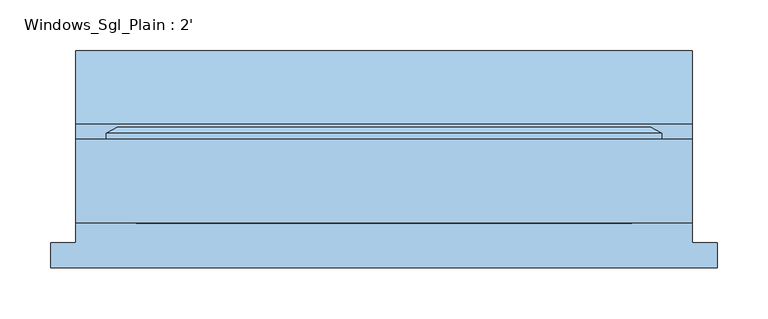
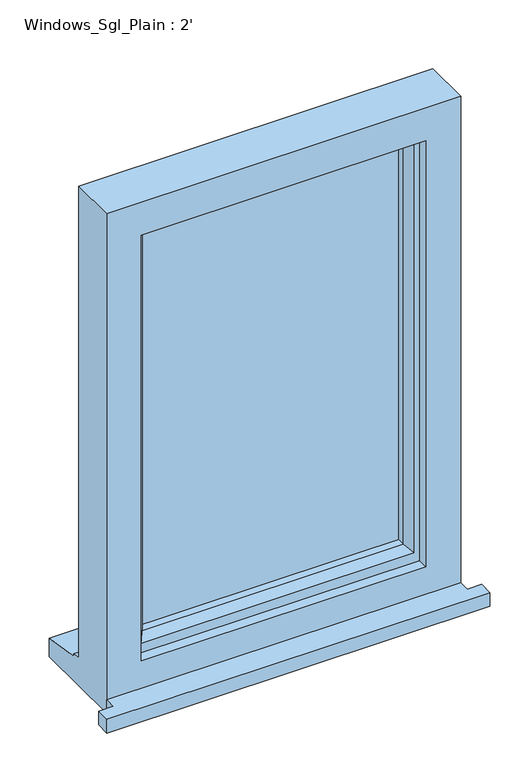
"""IFC4 building model written with IfcOpenShell, lengths in millimetres: window geometry, Windows_Sgl_Plain : 2'."""

from ifc_helpers import new_model, si_unit, frame, origin, place, context, project, spatial, polyline, outline, extrude, faceted_brep, source, transform, mapped, element, save


def windows_sgl_plain_2_be143095(model_context):
    return source(origin(), model_context, "Body", "SolidModel", [
        extrude(outline(polyline([(-329.8, -92.7434322), (-329.8, -67.7434322), (-304.8, -67.7434322), (-304.8, -48.3434322), (304.8, -48.3434322), (304.8, -67.7434322), (329.8, -67.7434322), (329.8, -92.7434322), (-329.8, -92.7434322)])), frame((0.0, 0.0, 1200.0), z_axis=(0.0, 0.0, 1.0), x_axis=(1.0, 0.0, 0.0)), (0.0, 0.0, 1.0), 25.0),
        faceted_brep([(-304.8, -48.3434322, 1200.0), (304.8, -48.3434322, 1200.0), (304.8, -48.3434322, 2110.0), (-304.8, -48.3434322, 2110.0), (-244.8, -48.3434322, 2050.0), (244.8, -48.3434322, 2050.0), (244.8, -48.3434322, 1275.0), (-244.8, -48.3434322, 1275.0), (-304.8, 34.6565678, 2110.0), (-304.8, 34.6565678, 1251.0), (-304.8, 49.6565678, 1249.68767), (-304.8, 49.6565678, 1244.7449676), (-304.8, 122.1565678, 1233.8088847), (-304.8, 122.1565678, 1200.0), (304.8, 34.6565678, 2110.0), (304.8, 34.6565678, 1251.0), (-264.8, 34.6565678, 2070.0), (-264.8, 34.6565678, 1263.0), (264.8, 34.6565678, 1263.0), (264.8, 34.6565678, 2070.0), (-264.8, -30.3434322, 2070.0), (-264.8, -30.3434322, 1263.0), (264.8, -30.3434322, 2070.0), (264.8, -30.3434322, 1263.0), (-244.8, -30.3434322, 2050.0), (-244.8, -30.3434322, 1275.0), (244.8, -30.3434322, 1275.0), (244.8, -30.3434322, 2050.0), (304.8, 122.1565678, 1200.0), (304.8, 122.1565678, 1233.8088847), (304.8, 49.6565678, 1244.7449676), (304.8, 49.6565678, 1249.68767)], [[[0, 1, 2, 3], [4, 5, 6, 7]], [[0, 3, 8, 9, 10, 11, 12, 13]], [[9, 8, 14, 15], [16, 17, 18, 19]], [[17, 16, 20, 21]], [[20, 22, 23, 21], [24, 25, 26, 27]], [[24, 4, 7, 25]], [[3, 2, 14, 8]], [[16, 19, 22, 20]], [[5, 4, 24, 27]], [[15, 14, 2, 1, 28, 29, 30, 31]], [[19, 18, 23, 22]], [[5, 27, 26, 6]], [[28, 1, 0, 13]], [[29, 28, 13, 12]], [[30, 29, 12, 11]], [[31, 30, 11, 10]], [[15, 31, 10, 9]], [[21, 23, 18, 17]], [[7, 6, 26, 25]]]),
        extrude(outline(polyline([(234.8, -1.3434322), (-234.8, -1.3434322), (-234.8, 22.6565678), (234.8, 22.6565678), (234.8, -1.3434322)])), frame((0.0, 0.0, 1293.0), z_axis=(0.0, 0.0, 1.0), x_axis=(1.0, 0.0, 0.0)), (0.0, 0.0, 1.0), 747.0),
        faceted_brep([(-274.8, 34.6565678, 2080.0), (-274.8, 40.4300705, 2080.0), (-274.8, 40.4300705, 1253.0), (-274.8, 34.6565678, 1253.0), (-264.8, -30.3434322, 2070.0), (-264.8, 34.6565678, 2070.0), (-264.8, 34.6565678, 1263.0), (-264.8, -30.3434322, 1263.0), (-224.8, -15.8505323, 2030.0), (-234.9480377, -30.3434322, 2040.1480377), (-234.9480377, -30.3434322, 1292.8519623), (-224.8, -15.8505323, 1303.0), (-224.8, -1.3434322, 2030.0), (-224.8, -1.3434322, 1303.0), (-234.8, 22.6565678, 2040.0), (-234.8, -1.3434322, 2040.0), (-234.8, -1.3434322, 1293.0), (-234.8, 22.6565678, 1293.0), (-224.8, 40.4300705, 2030.0), (-224.8, 22.6565678, 2030.0), (-224.8, 22.6565678, 1303.0), (-224.8, 40.4300705, 1303.0), (-242.2457548, 46.2035732, 2047.4457548), (-242.2457548, 46.2035732, 1285.5542452), (-264.0153903, 46.2035732, 2069.2153903), (-264.0153903, 46.2035732, 1263.7846097), (274.8, 40.4300705, 1253.0), (274.8, 34.6565678, 1253.0), (264.8, 34.6565678, 1263.0), (264.8, -30.3434322, 1263.0), (234.9480377, -30.3434322, 1292.8519623), (224.8, -15.8505323, 1303.0), (224.8, -1.3434322, 1303.0), (234.8, -1.3434322, 1293.0), (234.8, 22.6565678, 1293.0), (224.8, 22.6565678, 1303.0), (224.8, 40.4300705, 1303.0), (242.2457548, 46.2035732, 1285.5542452), (264.0153903, 46.2035732, 1263.7846097), (274.8, 40.4300705, 2080.0), (274.8, 34.6565678, 2080.0), (264.8, 34.6565678, 2070.0), (264.8, -30.3434322, 2070.0), (234.9480377, -30.3434322, 2040.1480377), (224.8, -15.8505323, 2030.0), (224.8, -1.3434322, 2030.0), (234.8, -1.3434322, 2040.0), (234.8, 22.6565678, 2040.0), (224.8, 22.6565678, 2030.0), (224.8, 40.4300705, 2030.0), (242.2457548, 46.2035732, 2047.4457548), (264.0153903, 46.2035732, 2069.2153903)], [[[0, 1, 2, 3]], [[4, 5, 6, 7]], [[8, 9, 10, 11]], [[12, 8, 11, 13]], [[14, 15, 16, 17]], [[18, 19, 20, 21]], [[22, 18, 21, 23]], [[1, 24, 25, 2]], [[3, 2, 26, 27]], [[7, 6, 28, 29]], [[11, 10, 30, 31]], [[13, 11, 31, 32]], [[17, 16, 33, 34]], [[21, 20, 35, 36]], [[23, 21, 36, 37]], [[2, 25, 38, 26]], [[27, 26, 39, 40]], [[29, 28, 41, 42]], [[31, 30, 43, 44]], [[32, 31, 44, 45]], [[34, 33, 46, 47]], [[36, 35, 48, 49]], [[37, 36, 49, 50]], [[26, 38, 51, 39]], [[40, 39, 1, 0]], [[3, 27, 40, 0], [5, 41, 28, 6]], [[42, 41, 5, 4]], [[7, 29, 42, 4], [9, 43, 30, 10]], [[44, 43, 9, 8]], [[45, 44, 8, 12]], [[15, 46, 33, 16], [13, 32, 45, 12]], [[47, 46, 15, 14]], [[17, 34, 47, 14], [19, 48, 35, 20]], [[49, 48, 19, 18]], [[50, 49, 18, 22]], [[24, 51, 38, 25], [23, 37, 50, 22]], [[39, 51, 24, 1]]]),
    ])


if __name__ == "__main__":
    model = new_model("IFC4")
    model_context = context("Model", 3, world=origin())
    ifc_project = project(units=[si_unit("LENGTHUNIT", "METRE", prefix="MILLI")], contexts=[model_context])
    site = spatial("IfcSite", under=ifc_project)
    building = spatial("IfcBuilding", under=site)
    placement = place(None, origin())
    windows_sgl_plain_2_shape = windows_sgl_plain_2_be143095(model_context)
    element("IfcWindow", 1, ObjectType="Windows_Sgl_Plain : 2'", at=placement, inside=building, context=model_context, shape_type="MappedRepresentation", body=[
        mapped(windows_sgl_plain_2_shape, transform((0.0, 0.0, 0.0), x_axis=(1.0, 0.0, 0.0), y_axis=(0.0, 1.0, 0.0), z_axis=(0.0, 0.0, 1.0))),
    ])
    save(model, "model.ifc")

# Revit data of these elements
# Type "Windows_Sgl_Plain : 2'"
#   Type Mark = "72"
#   Operation = "SinglePanel"
#   Construction Type Id = "SGL"
#   Manufacturer = "Revit"
#   Keynote = "L10"
#   Analytic Construction = "Large single-glazed windows"
#   Wrap Layers (Ext) from Ext = 102.5 mm
#   Wrap Layers (Int) from Ext = 177.5 mm
#   Window Board Projection = 25 mm
#   Window Board Extension = 25 mm
#   Visual Light Transmittance = 0.9
#   Solar Heat Gain Coefficient = 0.86
#   Rough Width = 609.6 mm
#   Rough Height = 910 mm
#   Height = 910 mm
#   Width = 609.6 mm
#   Heat Transfer Coefficient (U) = 5.5617 W/(m²·K)
#   Glazing Thickness = 24 mm
#   FrameOffset - External = 50 mm
#   Frame Depth = 65 mm
#   Default Head Height = 2110 mm
#   Cill Depth = 87.5 mm
#   Cavity Closer Width = 50 mm
#   Cavity Closer Offset from Ext = 102.5 mm
#   Cavity Closer Depth = 85 mm
#   Vis - Cavity Closers = yes
#   Define Thermal Properties by = 1
#   Material Trim = Window Frame
#   Material Glass = Glass
#   Material Frame = Window Frame
#   Wall Closure = (empty or 0)
# Element 1 (IfcWindow, "Windows_Sgl_Plain : 2'")
#   Materials on its faces: "Window Frame", "Glass"
# Materials
#   "Window Frame": colour RGB 249 249 249, transparency 0, Keynote = "L10", Cost = 0
#   "Glass": class "Glass", colour RGB 0 128 192, transparency 0.9, Description = "Soda Lime Glass", Cost = 0
